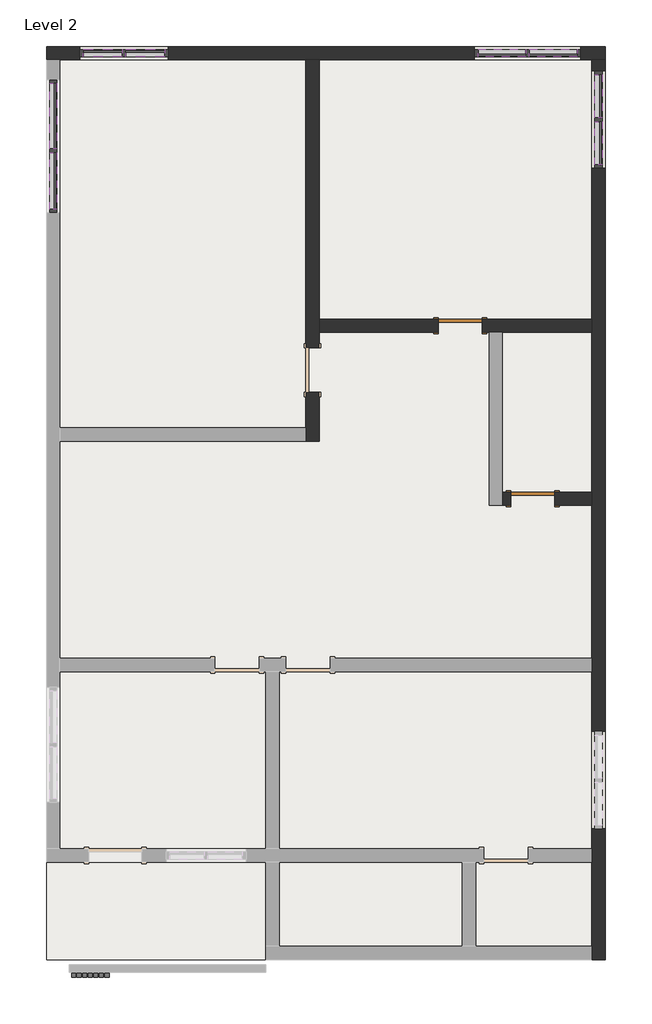
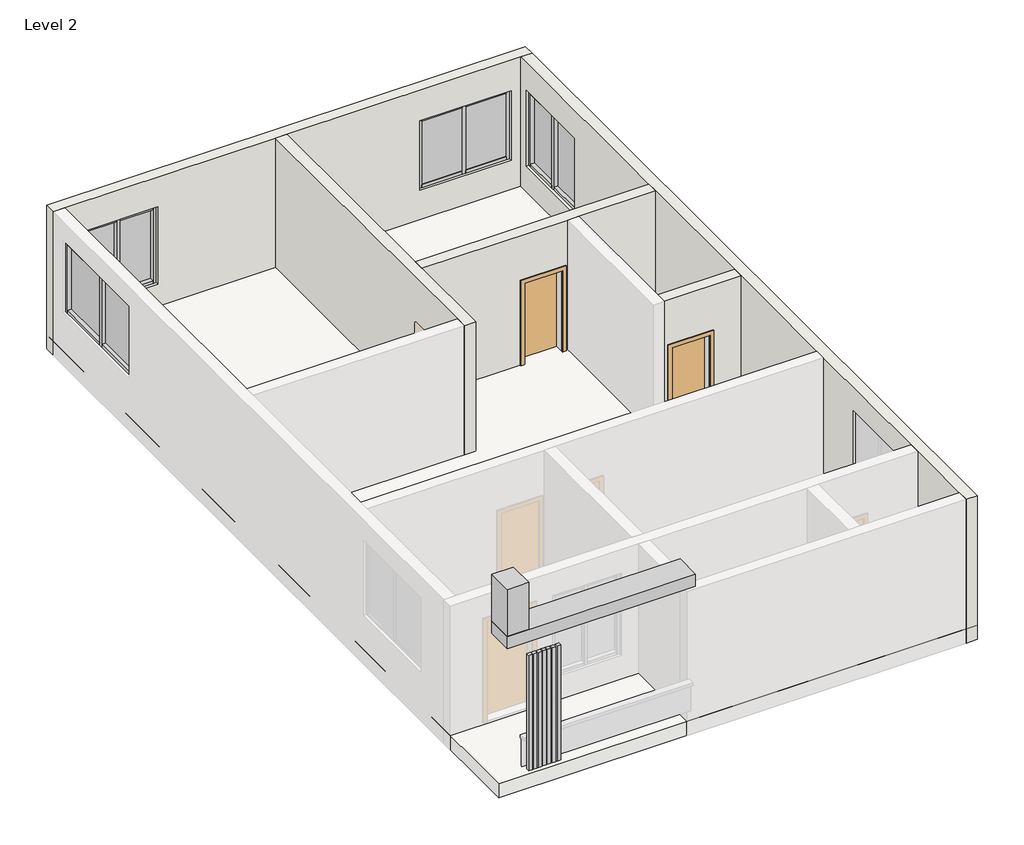
# One storey, part 2 of 2: 28 members, 8 plates, 5 walls, 2 doors, 1 proxy, 1 roof.
"""IFC4 building model written with IfcOpenShell, lengths in millimetres."""

from ifc_helpers import new_model, si_unit, frame, origin, place, context, project, spatial, polyline, outline, extrude, faceted_brep, transform, mapped, element, save
from components import generic_models_3_generic_models_3_6f6c0f21, door_85036156, door_a1484949, member_c33c434a, member_3a0a7659, member_780c4c5d, member_2dc5f12d, member_c17f1be2, member_7d2014ad, member_0bc7eccf, member_517f38dd, member_8f1a2d85, member_801a2072, member_e6b9f524, member_fae4a232, member_b4577db3, system_panel_glazed_945fd4ba, system_panel_glazed_44ef0770, system_panel_glazed_76c8377c, system_panel_glazed_53f2b764, system_panel_glazed_63a83b1f

model = new_model("IFC4")

# Units and contexts
model_context = context("Model", 3, world=origin())
ifc_project = project(units=[si_unit("LENGTHUNIT", "METRE", prefix="MILLI")], contexts=[model_context])

# Site, building, storey
site = spatial("IfcSite", under=ifc_project)
building = spatial("IfcBuilding", under=site)
storey = spatial("IfcBuildingStorey", under=building, Name="Level 2", Elevation=3048.0)

# Proxy
placement = place(None, origin())
generic_models_3_generic_models_3_shape = generic_models_3_generic_models_3_6f6c0f21(model_context)
element("IfcBuildingElementProxy", 1, Name="Generic Models 3 : Generic Models 3", ObjectType="Generic Models 3 : Generic Models 3", at=placement, inside=storey, context=model_context, shape_type="MappedRepresentation", body=[
    mapped(generic_models_3_generic_models_3_shape, transform((0.0, 0.0, 0.0), x_axis=(1.0, 0.0, 0.0), y_axis=(0.0, 1.0, 0.0), z_axis=(0.0, 0.0, 1.0))),
])

# Doors
door_shape = door_85036156(model_context)
element("IfcDoor", 2, ObjectType="Single-Flush : 30\" x 80\"", at=placement, inside=storey, context=model_context, shape_type="MappedRepresentation", body=[
    mapped(door_shape, transform((-7518.829521, -6416.0001929, 3048.0), x_axis=(-1.0, 0.0, 0.0), y_axis=(0.0, -1.0, 0.0), z_axis=(0.0, 0.0, 1.0))),
])
door_2_shape = door_a1484949(model_context)
element("IfcDoor", 3, ObjectType="Single-Flush : 30\" x 80\"", at=placement, inside=storey, context=model_context, shape_type="MappedRepresentation", body=[
    mapped(door_2_shape, transform((-8763.429521, -3444.2001929, 3048.0), x_axis=(1.0, 0.0, 0.0), y_axis=(0.0, 1.0, 0.0), z_axis=(0.0, 0.0, 1.0))),
])

# Members
member_shape = member_c33c434a(model_context)
element("IfcMember", 4, ObjectType="Rectangular Mullion : 2.5\" x 5\" rectangular", at=placement, inside=storey, context=model_context, shape_type="MappedRepresentation", body=[
    mapped(member_shape, transform((-14573.679521, 1242.0998071, 5462.9791667), x_axis=(0.0, 0.0, 1.0), y_axis=(0.0, -1.0, 0.0), z_axis=(1.0, 0.0, 0.0))),
])
element("IfcMember", 5, ObjectType="Rectangular Mullion : 2.5\" x 5\" rectangular", at=placement, inside=storey, context=model_context, shape_type="MappedRepresentation", body=[
    mapped(member_shape, transform((-13843.429521, 1242.0998071, 5462.9791667), x_axis=(0.0, 0.0, 1.0), y_axis=(0.0, -1.0, 0.0), z_axis=(1.0, 0.0, 0.0))),
])
element("IfcMember", 6, ObjectType="Rectangular Mullion : 2.5\" x 5\" rectangular", at=placement, inside=storey, context=model_context, shape_type="MappedRepresentation", body=[
    mapped(member_shape, transform((-14510.179521, 1242.0998071, 3828.7459672), x_axis=(0.0, 0.0, -1.0), y_axis=(0.0, -1.0, 0.0), z_axis=(-1.0, 0.0, 0.0))),
])
element("IfcMember", 7, ObjectType="Rectangular Mullion : 2.5\" x 5\" rectangular", at=placement, inside=storey, context=model_context, shape_type="MappedRepresentation", body=[
    mapped(member_shape, transform((-15240.429521, 1242.0998071, 3828.7459672), x_axis=(0.0, 0.0, -1.0), y_axis=(0.0, -1.0, 0.0), z_axis=(-1.0, 0.0, 0.0))),
])
member_2_shape = member_3a0a7659(model_context)
element("IfcMember", 8, ObjectType="Rectangular Mullion : 2.5\" x 5\" rectangular", at=placement, inside=storey, context=model_context, shape_type="MappedRepresentation", body=[
    mapped(member_2_shape, transform((-6388.529521, 130.8498071, 5506.346979), x_axis=(0.0, 0.0, 1.0), y_axis=(-1.0, 0.0, 0.0), z_axis=(0.0, -1.0, 0.0))),
])
element("IfcMember", 9, ObjectType="Rectangular Mullion : 2.5\" x 5\" rectangular", at=placement, inside=storey, context=model_context, shape_type="MappedRepresentation", body=[
    mapped(member_2_shape, transform((-6388.529521, -675.6001929, 5506.346979), x_axis=(0.0, 0.0, 1.0), y_axis=(-1.0, 0.0, 0.0), z_axis=(0.0, -1.0, 0.0))),
])
element("IfcMember", 10, ObjectType="Rectangular Mullion : 2.5\" x 5\" rectangular", at=placement, inside=storey, context=model_context, shape_type="MappedRepresentation", body=[
    mapped(member_2_shape, transform((-6388.529521, 67.3498071, 3895.1975587), x_axis=(0.0, 0.0, -1.0), y_axis=(-1.0, 0.0, 0.0), z_axis=(0.0, 1.0, 0.0))),
])
element("IfcMember", 11, ObjectType="Rectangular Mullion : 2.5\" x 5\" rectangular", at=placement, inside=storey, context=model_context, shape_type="MappedRepresentation", body=[
    mapped(member_2_shape, transform((-6388.529521, 873.7998071, 3895.1975587), x_axis=(0.0, 0.0, -1.0), y_axis=(-1.0, 0.0, 0.0), z_axis=(0.0, 1.0, 0.0))),
])
member_3_shape = member_780c4c5d(model_context)
element("IfcMember", 12, ObjectType="Rectangular Mullion : 2.5\" x 5\" rectangular", at=placement, inside=storey, context=model_context, shape_type="MappedRepresentation", body=[
    mapped(member_3_shape, transform((-6388.529521, 99.0998071, 3895.1975587), x_axis=(0.0, -1.0, 0.0), y_axis=(-1.0, 0.0, 0.0), z_axis=(0.0, 0.0, -1.0))),
])
member_4_shape = member_2dc5f12d(model_context)
element("IfcMember", 13, ObjectType="Rectangular Mullion : 2.5\" x 5\" rectangular", at=placement, inside=storey, context=model_context, shape_type="MappedRepresentation", body=[
    mapped(member_4_shape, transform((-6388.529521, 937.2998071, 5506.346979), x_axis=(0.0, 1.0, 0.0), y_axis=(-1.0, 0.0, 0.0), z_axis=(0.0, 0.0, 1.0))),
])
element("IfcMember", 14, ObjectType="Rectangular Mullion : 2.5\" x 5\" rectangular", at=placement, inside=storey, context=model_context, shape_type="MappedRepresentation", body=[
    mapped(member_4_shape, transform((-6388.529521, -739.1001929, 3895.1975587), x_axis=(0.0, -1.0, 0.0), y_axis=(-1.0, 0.0, 0.0), z_axis=(0.0, 0.0, -1.0))),
])
member_5_shape = member_c17f1be2(model_context)
element("IfcMember", 15, ObjectType="Rectangular Mullion : 2.5\" x 5\" rectangular", at=placement, inside=storey, context=model_context, shape_type="MappedRepresentation", body=[
    mapped(member_5_shape, transform((-7575.979521, 1242.0998071, 5447.7360356), x_axis=(0.0, 0.0, 1.0), y_axis=(0.0, 1.0, 0.0), z_axis=(-1.0, 0.0, 0.0))),
])
element("IfcMember", 16, ObjectType="Rectangular Mullion : 2.5\" x 5\" rectangular", at=placement, inside=storey, context=model_context, shape_type="MappedRepresentation", body=[
    mapped(member_5_shape, transform((-8458.629521, 1242.0998071, 5447.7360356), x_axis=(0.0, 0.0, 1.0), y_axis=(0.0, 1.0, 0.0), z_axis=(-1.0, 0.0, 0.0))),
])
member_6_shape = member_7d2014ad(model_context)
element("IfcMember", 17, ObjectType="Rectangular Mullion : 2.5\" x 5\" rectangular", at=placement, inside=storey, context=model_context, shape_type="MappedRepresentation", body=[
    mapped(member_6_shape, transform((-7607.729521, 1242.0998071, 3972.0301505), x_axis=(-1.0, 0.0, 0.0), y_axis=(0.0, 1.0, 0.0), z_axis=(0.0, 0.0, -1.0))),
])
element("IfcMember", 18, ObjectType="Rectangular Mullion : 2.5\" x 5\" rectangular", at=placement, inside=storey, context=model_context, shape_type="MappedRepresentation", body=[
    mapped(member_5_shape, transform((-7639.479521, 1242.0998071, 3972.0301505), x_axis=(0.0, 0.0, -1.0), y_axis=(0.0, 1.0, 0.0), z_axis=(1.0, 0.0, 0.0))),
])
element("IfcMember", 19, ObjectType="Rectangular Mullion : 2.5\" x 5\" rectangular", at=placement, inside=storey, context=model_context, shape_type="MappedRepresentation", body=[
    mapped(member_5_shape, transform((-6756.829521, 1242.0998071, 3972.0301505), x_axis=(0.0, 0.0, -1.0), y_axis=(0.0, 1.0, 0.0), z_axis=(1.0, 0.0, 0.0))),
])
member_7_shape = member_0bc7eccf(model_context)
element("IfcMember", 20, ObjectType="Rectangular Mullion : 2.5\" x 5\" rectangular", at=placement, inside=storey, context=model_context, shape_type="MappedRepresentation", body=[
    mapped(member_7_shape, transform((-8522.129521, 1242.0998071, 3972.0301505), x_axis=(-1.0, 0.0, 0.0), y_axis=(0.0, 1.0, 0.0), z_axis=(0.0, 0.0, -1.0))),
])
element("IfcMember", 21, ObjectType="Rectangular Mullion : 2.5\" x 5\" rectangular", at=placement, inside=storey, context=model_context, shape_type="MappedRepresentation", body=[
    mapped(member_7_shape, transform((-6693.329521, 1242.0998071, 5447.7360356), x_axis=(1.0, 0.0, 0.0), y_axis=(0.0, 1.0, 0.0), z_axis=(0.0, 0.0, 1.0))),
])
member_8_shape = member_517f38dd(model_context)
element("IfcMember", 22, ObjectType="Rectangular Mullion : 2.5\" x 5\" rectangular", at=placement, inside=storey, context=model_context, shape_type="MappedRepresentation", body=[
    mapped(member_8_shape, transform((-14541.929521, 1242.0998071, 3828.7459672), x_axis=(1.0, 0.0, 0.0), y_axis=(0.0, -1.0, 0.0), z_axis=(0.0, 0.0, -1.0))),
])
member_9_shape = member_8f1a2d85(model_context)
element("IfcMember", 23, ObjectType="Rectangular Mullion : 2.5\" x 5\" rectangular", at=placement, inside=storey, context=model_context, shape_type="MappedRepresentation", body=[
    mapped(member_9_shape, transform((-15303.929521, 1242.0998071, 5462.9791667), x_axis=(-1.0, 0.0, 0.0), y_axis=(0.0, -1.0, 0.0), z_axis=(0.0, 0.0, 1.0))),
])
element("IfcMember", 24, ObjectType="Rectangular Mullion : 2.5\" x 5\" rectangular", at=placement, inside=storey, context=model_context, shape_type="MappedRepresentation", body=[
    mapped(member_9_shape, transform((-13779.929521, 1242.0998071, 3828.7459672), x_axis=(1.0, 0.0, 0.0), y_axis=(0.0, -1.0, 0.0), z_axis=(0.0, 0.0, -1.0))),
])
member_10_shape = member_801a2072(model_context)
element("IfcMember", 25, ObjectType="Rectangular Mullion : 2.5\" x 5\" rectangular", at=placement, inside=storey, context=model_context, shape_type="MappedRepresentation", body=[
    mapped(member_10_shape, transform((-15761.129521, -1437.6001929, 5689.5924867), x_axis=(0.0, 0.0, 1.0), y_axis=(-1.0, 0.0, 0.0), z_axis=(0.0, -1.0, 0.0))),
])
member_11_shape = member_e6b9f524(model_context)
element("IfcMember", 26, ObjectType="Rectangular Mullion : 2.5\" x 5\" rectangular", at=placement, inside=storey, context=model_context, shape_type="MappedRepresentation", body=[
    mapped(member_11_shape, transform((-15761.129521, -402.5501929, 5689.5924867), x_axis=(0.0, 0.0, 1.0), y_axis=(-1.0, 0.0, 0.0), z_axis=(0.0, -1.0, 0.0))),
])
member_12_shape = member_fae4a232(model_context)
element("IfcMember", 27, ObjectType="Rectangular Mullion : 2.5\" x 5\" rectangular", at=placement, inside=storey, context=model_context, shape_type="MappedRepresentation", body=[
    mapped(member_12_shape, transform((-15761.129521, -434.3001929, 4168.4028546), x_axis=(0.0, -1.0, 0.0), y_axis=(-1.0, 0.0, 0.0), z_axis=(0.0, 0.0, -1.0))),
])
element("IfcMember", 28, ObjectType="Rectangular Mullion : 2.5\" x 5\" rectangular", at=placement, inside=storey, context=model_context, shape_type="MappedRepresentation", body=[
    mapped(member_10_shape, transform((-15761.129521, -466.0501929, 4168.4028546), x_axis=(0.0, 0.0, -1.0), y_axis=(-1.0, 0.0, 0.0), z_axis=(0.0, 1.0, 0.0))),
])
element("IfcMember", 29, ObjectType="Rectangular Mullion : 2.5\" x 5\" rectangular", at=placement, inside=storey, context=model_context, shape_type="MappedRepresentation", body=[
    mapped(member_11_shape, transform((-15761.129521, 721.3998071, 4168.4028546), x_axis=(0.0, 0.0, -1.0), y_axis=(-1.0, 0.0, 0.0), z_axis=(0.0, 1.0, 0.0))),
])
member_13_shape = member_b4577db3(model_context)
element("IfcMember", 30, ObjectType="Rectangular Mullion : 2.5\" x 5\" rectangular", at=placement, inside=storey, context=model_context, shape_type="MappedRepresentation", body=[
    mapped(member_13_shape, transform((-15761.129521, -1501.1001929, 4168.4028546), x_axis=(0.0, -1.0, 0.0), y_axis=(-1.0, 0.0, 0.0), z_axis=(0.0, 0.0, -1.0))),
])
element("IfcMember", 31, ObjectType="Rectangular Mullion : 2.5\" x 5\" rectangular", at=placement, inside=storey, context=model_context, shape_type="MappedRepresentation", body=[
    mapped(member_13_shape, transform((-15761.129521, 784.8998071, 5689.5924867), x_axis=(0.0, 1.0, 0.0), y_axis=(-1.0, 0.0, 0.0), z_axis=(0.0, 0.0, 1.0))),
])

# Plates
system_panel_glazed_shape = system_panel_glazed_945fd4ba(model_context)
element("IfcPlate", 32, ObjectType="System Panel : Glazed", at=placement, inside=storey, context=model_context, shape_type="MappedRepresentation", body=[
    mapped(system_panel_glazed_shape, transform((-6388.529521, 502.3248071, 3958.6975587), x_axis=(0.0, -1.0, 0.0), y_axis=(1.0, 0.0, 0.0), z_axis=(0.0, 0.0, 1.0))),
])
element("IfcPlate", 33, ObjectType="System Panel : Glazed", at=placement, inside=storey, context=model_context, shape_type="MappedRepresentation", body=[
    mapped(system_panel_glazed_shape, transform((-6388.529521, -304.1251929, 3958.6975587), x_axis=(0.0, -1.0, 0.0), y_axis=(1.0, 0.0, 0.0), z_axis=(0.0, 0.0, 1.0))),
])
system_panel_glazed_2_shape = system_panel_glazed_44ef0770(model_context)
element("IfcPlate", 34, ObjectType="System Panel : Glazed", at=placement, inside=storey, context=model_context, shape_type="MappedRepresentation", body=[
    mapped(system_panel_glazed_2_shape, transform((-7166.404521, 1242.0998071, 4035.5301505), x_axis=(-1.0, 0.0, 0.0), y_axis=(0.0, -1.0, 0.0), z_axis=(0.0, 0.0, 1.0))),
])
element("IfcPlate", 35, ObjectType="System Panel : Glazed", at=placement, inside=storey, context=model_context, shape_type="MappedRepresentation", body=[
    mapped(system_panel_glazed_2_shape, transform((-8049.054521, 1242.0998071, 4035.5301505), x_axis=(-1.0, 0.0, 0.0), y_axis=(0.0, -1.0, 0.0), z_axis=(0.0, 0.0, 1.0))),
])
system_panel_glazed_3_shape = system_panel_glazed_76c8377c(model_context)
element("IfcPlate", 36, ObjectType="System Panel : Glazed", at=placement, inside=storey, context=model_context, shape_type="MappedRepresentation", body=[
    mapped(system_panel_glazed_3_shape, transform((-14907.054521, 1242.0998071, 3892.2459672), x_axis=(1.0, 0.0, 0.0), y_axis=(0.0, 1.0, 0.0), z_axis=(0.0, 0.0, 1.0))),
])
element("IfcPlate", 37, ObjectType="System Panel : Glazed", at=placement, inside=storey, context=model_context, shape_type="MappedRepresentation", body=[
    mapped(system_panel_glazed_3_shape, transform((-14176.804521, 1242.0998071, 3892.2459672), x_axis=(1.0, 0.0, 0.0), y_axis=(0.0, 1.0, 0.0), z_axis=(0.0, 0.0, 1.0))),
])
system_panel_glazed_4_shape = system_panel_glazed_53f2b764(model_context)
element("IfcPlate", 38, ObjectType="System Panel : Glazed", at=placement, inside=storey, context=model_context, shape_type="MappedRepresentation", body=[
    mapped(system_panel_glazed_4_shape, transform((-15761.129521, 159.4248071, 4231.9028546), x_axis=(0.0, -1.0, 0.0), y_axis=(1.0, 0.0, 0.0), z_axis=(0.0, 0.0, 1.0))),
])
system_panel_glazed_5_shape = system_panel_glazed_63a83b1f(model_context)
element("IfcPlate", 39, ObjectType="System Panel : Glazed", at=placement, inside=storey, context=model_context, shape_type="MappedRepresentation", body=[
    mapped(system_panel_glazed_5_shape, transform((-15761.129521, -951.8251929, 4231.9028546), x_axis=(0.0, -1.0, 0.0), y_axis=(1.0, 0.0, 0.0), z_axis=(0.0, 0.0, 1.0))),
])

# Roof
element("IfcRoof", 40, ObjectType="Generic - 12\"", at=placement, inside=storey, context=model_context, shape_type="SweptSolid", body=[
    extrude(outline(polyline([(-15875.429521, 1356.3998071), (-6274.229521, 1356.3998071), (-6274.229521, -14340.8001929), (-15875.429521, -14340.8001929), (-15875.429521, 1356.3998071)])), frame((0.0, 0.0, 3048.0), z_axis=(0.0, 0.0, 1.0), x_axis=(1.0, 0.0, 0.0)), (0.0, 0.0, 1.0), 304.8),
])

# Walls
element("IfcWall", 41, ObjectType="9\"", at=placement, inside=storey, context=model_context, shape_type="Brep", body=[
    faceted_brep([(-15875.429521, 1127.7998071, 3048.0), (-15646.829521, 1127.7998071, 3048.0), (-11417.729521, 1127.7998071, 3048.0), (-11189.129521, 1127.7998071, 3048.0), (-6502.829521, 1127.7998071, 3048.0), (-6274.229521, 1127.7998071, 3048.0), (-6274.229521, 1127.7998071, 6096.0), (-6502.829521, 1127.7998071, 6096.0), (-11189.129521, 1127.7998071, 6096.0), (-11417.729521, 1127.7998071, 6096.0), (-15646.829521, 1127.7998071, 6096.0), (-15875.429521, 1127.7998071, 6096.0), (-15303.929521, 1127.7998071, 3828.7459672), (-15303.929521, 1127.7998071, 5462.9791667), (-13779.929521, 1127.7998071, 5462.9791667), (-13779.929521, 1127.7998071, 3828.7459672), (-6693.329521, 1127.7998071, 5447.7360356), (-6693.329521, 1127.7998071, 3972.0301505), (-8522.129521, 1127.7998071, 3972.0301505), (-8522.129521, 1127.7998071, 5447.7360356), (-6274.229521, 1356.3998071, 3048.0), (-15875.429521, 1356.3998071, 3048.0), (-15875.429521, 1356.3998071, 6096.0), (-6274.229521, 1356.3998071, 6096.0), (-15303.929521, 1356.3998071, 5462.9791667), (-15303.929521, 1356.3998071, 3828.7459672), (-13779.929521, 1356.3998071, 3828.7459672), (-13779.929521, 1356.3998071, 5462.9791667), (-6693.329521, 1356.3998071, 3972.0301505), (-6693.329521, 1356.3998071, 5447.7360356), (-8522.129521, 1356.3998071, 5447.7360356), (-8522.129521, 1356.3998071, 3972.0301505)], [[[0, 1, 2, 3, 4, 5, 6, 7, 8, 9, 10, 11], [12, 13, 14, 15], [16, 17, 18, 19]], [[20, 21, 22, 23], [24, 25, 26, 27], [28, 29, 30, 31]], [[5, 4, 3, 2, 1, 0, 21, 20]], [[11, 10, 9, 8, 7, 6, 23, 22]], [[6, 5, 20, 23]], [[0, 11, 22, 21]], [[12, 25, 24, 13]], [[13, 24, 27, 14]], [[14, 27, 26, 15]], [[25, 12, 15, 26]], [[28, 17, 16, 29]], [[29, 16, 19, 30]], [[18, 31, 30, 19]], [[17, 28, 31, 18]]]),
])
element("IfcWall", 42, ObjectType="9\"", at=placement, inside=storey, context=model_context, shape_type="Brep", body=[
    faceted_brep([(-6502.829521, 1127.7998071, 3048.0), (-6502.829521, -3329.9001929, 3048.0), (-6502.829521, -3558.5001929, 3048.0), (-6502.829521, -6301.7001929, 3048.0), (-6502.829521, -6530.3001929, 3048.0), (-6502.829521, -9159.2001929, 3048.0), (-6502.829521, -9387.8001929, 3048.0), (-6502.829521, -12435.8001929, 3048.0), (-6502.829521, -12664.4001929, 3048.0), (-6502.829521, -14112.2001929, 3048.0), (-6502.829521, -14340.8001929, 3048.0), (-6502.829521, -14340.8001929, 6096.0), (-6502.829521, -14112.2001929, 6096.0), (-6502.829521, -12664.4001929, 6096.0), (-6502.829521, -12435.8001929, 6096.0), (-6502.829521, -9387.8001929, 6096.0), (-6502.829521, -9159.2001929, 6096.0), (-6502.829521, -6530.3001929, 6096.0), (-6502.829521, -6301.7001929, 6096.0), (-6502.829521, -3558.5001929, 6096.0), (-6502.829521, -3329.9001929, 6096.0), (-6502.829521, 1127.7998071, 6096.0), (-6502.829521, -12092.9001929, 5595.2359655), (-6502.829521, -12092.9001929, 3941.2993086), (-6502.829521, -10416.5001929, 3941.2993086), (-6502.829521, -10416.5001929, 5595.2359655), (-6502.829521, 937.2998071, 3895.1975587), (-6502.829521, 937.2998071, 5506.346979), (-6502.829521, -739.1001929, 5506.346979), (-6502.829521, -739.1001929, 3895.1975587), (-6274.229521, -14340.8001929, 3048.0), (-6274.229521, 1127.7998071, 3048.0), (-6274.229521, 1127.7998071, 6096.0), (-6274.229521, -14340.8001929, 6096.0), (-6274.229521, -12092.9001929, 3941.2993086), (-6274.229521, -12092.9001929, 5595.2359655), (-6274.229521, -10416.5001929, 5595.2359655), (-6274.229521, -10416.5001929, 3941.2993086), (-6274.229521, 937.2998071, 5506.346979), (-6274.229521, 937.2998071, 3895.1975587), (-6274.229521, -739.1001929, 3895.1975587), (-6274.229521, -739.1001929, 5506.346979)], [[[0, 1, 2, 3, 4, 5, 6, 7, 8, 9, 10, 11, 12, 13, 14, 15, 16, 17, 18, 19, 20, 21], [22, 23, 24, 25], [26, 27, 28, 29]], [[30, 31, 32, 33], [34, 35, 36, 37], [38, 39, 40, 41]], [[10, 9, 8, 7, 6, 5, 4, 3, 2, 1, 0, 31, 30]], [[21, 20, 19, 18, 17, 16, 15, 14, 13, 12, 11, 33, 32]], [[0, 21, 32, 31]], [[11, 10, 30, 33]], [[34, 23, 22, 35]], [[35, 22, 25, 36]], [[36, 25, 24, 37]], [[23, 34, 37, 24]], [[26, 39, 38, 27]], [[27, 38, 41, 28]], [[40, 29, 28, 41]], [[39, 26, 29, 40]]]),
])
element("IfcWall", 43, ObjectType="9\"", at=placement, inside=storey, context=model_context, shape_type="Brep", body=[
    faceted_brep([(-11417.729521, 1127.7998071, 3048.0), (-11417.729521, -3825.2001929, 3048.0), (-11417.729521, -3825.2001929, 5080.0), (-11417.729521, -4587.2001929, 5080.0), (-11417.729521, -4587.2001929, 3048.0), (-11417.729521, -5196.8001929, 3048.0), (-11417.729521, -5425.4001929, 3048.0), (-11417.729521, -5425.4001929, 6096.0), (-11417.729521, -5196.8001929, 6096.0), (-11417.729521, 1127.7998071, 6096.0), (-11189.129521, -3825.2001929, 5080.0), (-11189.129521, -3825.2001929, 3048.0), (-11189.129521, -3558.5001929, 3048.0), (-11189.129521, -3329.9001929, 3048.0), (-11189.129521, 1127.7998071, 3048.0), (-11189.129521, 1127.7998071, 6096.0), (-11189.129521, -3329.9001929, 6096.0), (-11189.129521, -3558.5001929, 6096.0), (-11189.129521, -5425.4001929, 6096.0), (-11189.129521, -5425.4001929, 3048.0), (-11189.129521, -4587.2001929, 3048.0), (-11189.129521, -4587.2001929, 5080.0)], [[[0, 1, 2, 3, 4, 5, 6, 7, 8, 9]], [[10, 11, 12, 13, 14, 15, 16, 17, 18, 19, 20, 21]], [[20, 19, 6, 5, 4]], [[14, 13, 12, 11, 1, 0]], [[9, 8, 7, 18, 17, 16, 15]], [[0, 9, 15, 14]], [[7, 6, 19, 18]], [[2, 1, 11, 10]], [[3, 2, 10, 21]], [[4, 3, 21, 20]]]),
])
element("IfcWall", 44, ObjectType="9\"", at=placement, inside=storey, context=model_context, shape_type="Brep", body=[
    faceted_brep([(-8382.429521, -3558.5001929, 5080.0), (-8382.429521, -3558.5001929, 3048.0), (-8268.129521, -3558.5001929, 3048.0), (-8039.529521, -3558.5001929, 3048.0), (-6502.829521, -3558.5001929, 3048.0), (-6502.829521, -3558.5001929, 6096.0), (-8039.529521, -3558.5001929, 6096.0), (-8268.129521, -3558.5001929, 6096.0), (-11189.129521, -3558.5001929, 6096.0), (-11189.129521, -3558.5001929, 3048.0), (-9144.429521, -3558.5001929, 3048.0), (-9144.429521, -3558.5001929, 5080.0), (-6502.829521, -3329.9001929, 3048.0), (-8382.429521, -3329.9001929, 3048.0), (-8382.429521, -3329.9001929, 5080.0), (-9144.429521, -3329.9001929, 5080.0), (-9144.429521, -3329.9001929, 3048.0), (-11189.129521, -3329.9001929, 3048.0), (-11189.129521, -3329.9001929, 6096.0), (-6502.829521, -3329.9001929, 6096.0)], [[[0, 1, 2, 3, 4, 5, 6, 7, 8, 9, 10, 11]], [[12, 13, 14, 15, 16, 17, 18, 19]], [[10, 9, 17, 16]], [[4, 3, 2, 1, 13, 12]], [[8, 7, 6, 5, 19, 18]], [[5, 4, 12, 19]], [[9, 8, 18, 17]], [[14, 13, 1, 0]], [[15, 14, 0, 11]], [[16, 15, 11, 10]]]),
])
element("IfcWall", 45, ObjectType="9\"", at=placement, inside=storey, context=model_context, shape_type="SweptSolid", body=[
    extrude(outline(polyline([(3048.0, -8039.529521), (3048.0, -7899.829521), (5080.0, -7899.829521), (5080.0, -7137.829521), (3048.0, -7137.829521), (3048.0, -6502.829521), (6096.0, -6502.829521), (6096.0, -8039.529521), (3048.0, -8039.529521)])), frame((0.0, -6530.3001929, 0.0), z_axis=(0.0, 1.0, 0.0), x_axis=(0.0, 0.0, 1.0)), (0.0, 0.0, 1.0), 228.6),
])

save(model, "model.ifc")

# Revit data of these elements
# Type "Single-Flush : 30\" x 80\""
#   Type Mark = "5"
#   Construction Type Id = "MDOOR"
#   Assembly Code = "C1020"
#   Analytic Construction = "Metal"
#   Thickness = 0' - 2"
#   Heat Transfer Coefficient (U) = 0.651978 BTU/(h·ft²·°F)
#   Height = 6' - 8"
#   Trim Projection Ext = 0' - 1"
#   Trim Projection Int = 0' - 1"
#   Trim Width = 0' - 3"
#   Width = 2' - 6"
#   Define Thermal Properties by = 1
#   Define Thermal Properties by = 1
#   Door Material = Door - Panel
#   Frame Material = Door - Frame
#   Visual Light Transmittance = 0
#   Solar Heat Gain Coefficient = 0
#   Function = (empty or 0)
#   Wall Closure = (empty or 0)
# Type "Rectangular Mullion : 2.5\" x 5\" rectangular"
#   built-in parameter 1007304 = 0.416667 (stored number, unit not read)
#   built-in parameter 1007301 = 0.104167 (stored number, unit not read)
#   built-in parameter 1007300 = 0.104167 (stored number, unit not read)
# Type "System Panel : Glazed"
#   Construction Type Id = "GSP4R"
#   Analytic Construction = "1/8 in Pilkington single glazing"
#   Visual Light Transmittance = 0.9
#   Solar Heat Gain Coefficient = 0.86
#   Heat Transfer Coefficient (U) = 1.18115 BTU/(h·ft²·°F)
#   Define Thermal Properties by = 1
# Type "Generic - 12\""
#   Assembly Code = "B1020"
#   Layers, outside or top first: 1' - 0" no material (function 1)
# Type "9\""
#   Assembly Code = "B2010"
#   Layers, outside or top first: 0' - 9" no material (function 1)
# Element 1 (IfcBuildingElementProxy, "Generic Models 3 : Generic Models 3")
#   Phase Created = New Construction
# Elements 2, 3 (IfcDoor, "Single-Flush : 30\" x 80\"")
#   Phase Created = New Construction
#   Materials on its faces: "Door - Frame", "Door - Panel"
# Elements 4, 5, 6, 7, 8, 9, 10, 11, 12, 13, 14, 15, 16, 17, 18, 19, 20, 21, 22, 23, 24, 25, 26, 27, 28, 29, 30, 31 (IfcMember, "Rectangular Mullion : 2.5\" x 5\" rectangular")
#   Phase Created = New Construction
#   Materials on its faces: "Aluminum"
# Elements 32, 33, 34, 35, 36, 37, 38, 39 (IfcPlate, "System Panel : Glazed")
#   Phase Created = New Construction
#   Materials on its faces: "Glass"
# Element 40 (IfcRoof, "Generic - 12\"")
#   built-in parameter 1001705 = 11 (stored number, unit not read)
#   built-in parameter 1001710 = 33615
#   Phase Created = New Construction
#   Materials on its faces: "Default Roof"
# Elements 41, 42, 43, 44, 45 (IfcWall, "9\"")
#   Top Offset = 0' - 0"
#   Base Offset = 0' - 0"
#   Unconnected Height = 10' - 0"
#   wall height = 10' - 0"
#   Phase Created = New Construction
#   Base Constraint = Level 2
#   Materials on its faces: "Default Wall"
# Materials
#   "Door - Panel": class "Wood", colour RGB 210 159 95, transparency 0, Cost = 0
#   "Door - Frame": colour RGB 118 70 51, transparency 0, Cost = 0
#   "Aluminum": class "Metal", colour RGB 247 247 247, transparency 0, Description = "Aluminum 6061", Cost = 0
#   "Glass": class "Glass", colour RGB 0 128 192, transparency 0.75, Description = "Soda Lime Glass", Cost = 0
#   "Default Roof": colour RGB 88 101 114, transparency 0, Cost = 0
#   "Default Wall": colour RGB 128 128 128, transparency 0, Cost = 0
